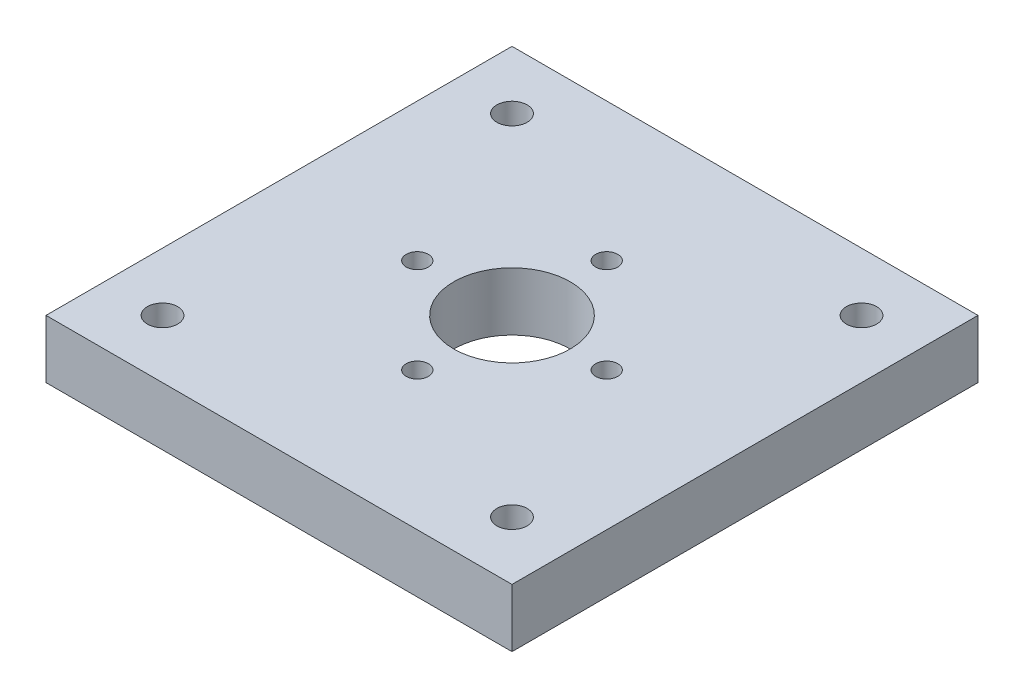
SolidWorks part; units mm, degrees
material "Plain Carbon Steel"
ref_plane "Front Plane" through (0, 0, 0) normal (0, 0, 1) x (1, 0, 0)
ref_plane "Top Plane" through (0, 0, 0) normal (0, 1, 0) x (1, 0, 0)
ref_plane "Right Plane" through (0, 0, 0) normal (1, 0, 0) x (0, 0, -1)
sketch "Base Plate Profile" plane through (0, 0, 0) normal (0, 1, 0) x (1, 0, 0)
  line L0 (-243.129, 0) -> (350.5285, 0) construction
  line L1 (-200, -200) -> (200, -200)
  line L2 (-200, -200) -> (-200, 200)
  line L3 (-200, 200) -> (200, 200)
  line L4 (200, -200) -> (200, 200)
  line L5 (-200, -200) -> (200, 200) construction
  line L6 (-200, 200) -> (200, -200) construction
  line L7 (0, -250.74) -> (0, 306.5539) construction
  circle A0 centre (0, 0) radius 50
  circle A1 centre (150, 150) radius 13
  circle A2 centre (-150, 150) radius 13
  circle A3 centre (150, -150) radius 13
  circle A4 centre (-150, -150) radius 13
  circle A5 centre (0, 0) radius 81.3 construction
  circle A6 centre (0, 81.3) radius 9.5
  circle A7 centre (0, -81.3) radius 9.5
  circle A8 centre (-81.3, 0) radius 9.5
  circle A9 centre (81.3, 0) radius 9.5
  point P0 (0, 0)
  dimension "D3" = 100
  dimension "D4" = 26
  dimension "D6" = 19
  dimension "162.6" = 162.6
  dimension "D7" = 19
  dimension "D1" = 400
  dimension "D2" = 400
  dimension "D5" = 150
extrude "Base Plate 400x400x50" add sketch "Base Plate Profile" along normal mid plane 50
